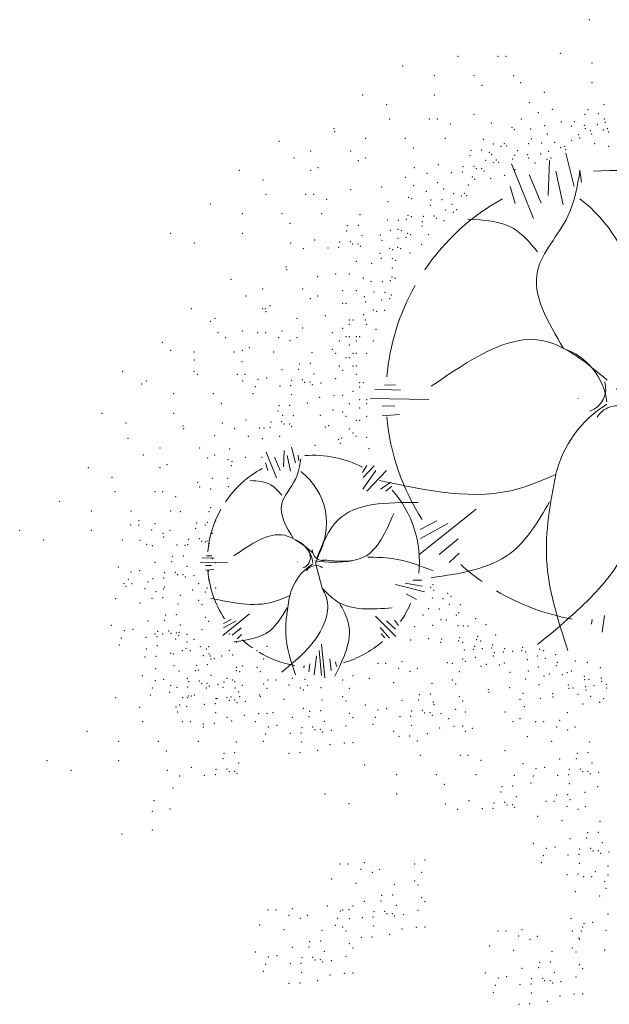
# Model space of a CAD drawing. Units: inches. Extents: x 1239 to 2276906, y 2273 to 321338.
# Tile 22 of 23: x 2267886 to 2272170, y 313785 to 320943. Entities that reach past the tile are written whole.
import ezdxf

# ---------------------------------------------------------------- set-up
doc = ezdxf.new("R2010")
doc.units = ezdxf.units.IN
doc.layers.add('L-PLNT', color=94, linetype='Continuous', lineweight=13)

# ---------------------------------------------------------------- blocks, each defined once
blk = doc.blocks.new('A$C30B31857')
for p, q in [((2.9834, 4.9924), (2.9378, 5.171)), ((2.7648, 4.82), (2.6466, 5.1137)), ((2.8434, 4.944), (2.8514, 5.1313)), ((2.8062, 4.9013), (2.7413, 5.0568)), ((2.9247, 4.894), (2.8853, 5.0751)), ((3.0223, 5.0135), (3.0144, 5.0799)), ((2.6661, 4.9009), (2.6393, 4.9915)), ((1.9621, 3.9222), (2.0223, 3.9241)), ((1.9103, 3.9012), (2.0497, 3.8956)), ((1.8883, 3.8498), (2.2022, 3.8449)), ((1.9494, 3.7571), (2.0441, 3.7647)), ((1.9499, 3.8105), (2.0188, 3.8098)), ((1.3819, 3.4241), (1.3265, 3.5618)), ((1.4188, 3.4822), (1.4225, 3.57)), ((1.4844, 3.5049), (1.463, 3.5887)), ((1.3356, 3.462), (1.3231, 3.5045)), ((1.4013, 3.4622), (1.3709, 3.5351)), ((1.4568, 3.4588), (1.4384, 3.5437)), ((1.5026, 3.5148), (1.4989, 3.546)), ((1.8439, 3.4518), (1.8684, 3.4899)), ((1.847, 3.3622), (1.9166, 3.4632)), ((1.8485, 3.4247), (1.9067, 3.4887)), ((1.868, 3.352), (1.973, 3.4627)), ((1.9418, 3.3622), (1.9966, 3.3999)), ((1.9699, 3.3518), (2.0024, 3.3789)), ((2.1467, 3.0086), (2.4563, 3.255)), ((2.1542, 3.1461), (2.2449, 3.1926)), ((2.1561, 3.097), (2.3032, 3.1772)), ((1.594, 2.9655), (1.6381, 3.0897)), ((2.2561, 3.01), (2.3583, 3.095)), ((0.971, 2.9694), (1.1182, 2.967)), ((0.9814, 2.9934), (1.0467, 2.9908)), ((1.0056, 3.0033), (1.0339, 3.0042)), ((2.3116, 2.9682), (2.3637, 3.0175)), ((0.9997, 2.9259), (1.0441, 2.9295)), ((0.9999, 2.9509), (1.0322, 2.9506)), ((1.5913, 2.9655), (1.6271, 2.8302)), ((2.1639, 2.8721), (2.1155, 2.8726)), ((2.1774, 2.8094), (2.0226, 2.8493)), ((2.1665, 2.8407), (2.0739, 2.8568)), ((2.1347, 2.7684), (2.0785, 2.7983)), ((1.0922, 2.575), (1.2373, 2.6905)), ((1.0957, 2.6395), (1.1382, 2.6613)), ((1.0966, 2.6164), (1.1655, 2.6541)), ((2.0239, 2.569), (1.9137, 2.6778)), ((2.0211, 2.6094), (1.9743, 2.6542)), ((2.0385, 2.6282), (2.0167, 2.6578)), ((3.0763, 2.6357), (3.0809, 2.6614)), ((3.1343, 2.5921), (3.1456, 2.6823)), ((1.1434, 2.5757), (1.1913, 2.6155)), ((1.9903, 2.5593), (1.9397, 2.6182)), ((1.1695, 2.5561), (1.1939, 2.5792)), ((1.9642, 2.5615), (1.9442, 2.5828)), ((1.6235, 2.359), (1.6107, 2.4933)), ((1.6415, 2.3458), (1.624, 2.5274)), ((1.584, 2.3634), (1.5971, 2.4652)), ((1.675, 2.3867), (1.6687, 2.4492)), ((1.5279, 2.4002), (1.5301, 2.4123)), ((1.5551, 2.3798), (1.5604, 2.4221)), ((1.7046, 2.4077), (1.6996, 2.4328))]:
    blk.add_line(p, q)
for centre, radius, start, end in [((3.1873, 3.861), 1.217, 62.402, 94.6709), ((3.1873, 3.861), 1.217, 118.935, 145.868), ((2.5377, 4.3028), 0.7844, 329.0782, 52.6009), ((3.1873, 3.861), 1.217, 150.5954, 174.9599), ((2.8122, 3.7899), 0.3494, 6.8841, 70.9351), ((3.0261, 3.9032), 0.1272, 289.2154, 17.1317), ((3.4797, 3.2971), 0.6129, 121.5433, 166.6017), ((3.1338, 3.8505), 0.1272, 179.4366, 180.2669), ((3.2157, 3.6838), 0.1272, 52.7337, 148.3189), ((3.1873, 3.861), 1.217, 185.1155, 212.961), ((1.58, 2.9746), 0.5705, 62.402, 94.6709), ((1.58, 2.9746), 0.5705, 118.935, 145.868), ((1.2979, 3.1775), 0.353, 329.0782, 52.6009), ((1.58, 2.9746), 0.5705, 353.5054, 42.0912), ((1.58, 2.9746), 0.5705, 150.5954, 174.9599), ((1.4214, 2.9466), 0.1572, 6.8841, 70.9351), ((1.633, 3.0374), 0.0596, 180.2669, 289.2154), ((1.5549, 2.9697), 0.0596, 179.4366, 180.2669), ((1.5044, 2.9943), 0.0596, 289.2154, 17.1317), ((1.6891, 3.6438), 0.6749, 261.4278, 278.5722), ((1.58, 2.9746), 0.5705, 185.1155, 212.961), ((1.7218, 2.7249), 0.2758, 121.5433, 166.6017), ((1.5933, 2.8915), 0.0596, 52.7337, 148.3189), ((3.1873, 3.861), 1.217, 227.9939, 234.9207), ((3.1873, 3.861), 1.217, 239.2549, 259.861), ((1.58, 2.9746), 0.5705, 325.3181, 336.4192), ((1.58, 2.9746), 0.5705, 227.9939, 234.9207), ((1.58, 2.9746), 0.5705, 286.5005, 310.702), ((1.58, 2.9746), 0.5705, 239.2549, 259.861)]:
    blk.add_arc(centre, radius, start, end)
for points, knots in [([(2.9263, 4.1201), (2.841, 4.2637), (2.6905, 4.5171), (2.9681, 4.7985), (3.0006, 4.9937), (3.0146, 5.0775)], [0, 0, 0, 0, 0.440566, 0.777274, 1.031196, 1.031196, 1.031196, 1.031196]), ([(2.7862, 4.6403), (2.7459, 4.6888), (2.6503, 4.8039), (2.4983, 4.8115), (2.4103, 4.8158)], [0, 0, 0, 0, 0.1819315, 0.4317682, 0.4317682, 0.4317682, 0.4317682]), ([(3.1616, 3.9488), (3.0492, 4.0429), (2.7553, 4.2891), (2.4209, 4.0585), (2.2144, 3.9161)], [0, 0, 0, 0, 0.40354, 1.055721, 1.055721, 1.055721, 1.055721]), ([(1.4728, 3.0952), (1.4344, 3.1599), (1.3667, 3.2739), (1.4916, 3.4005), (1.5062, 3.4883), (1.5125, 3.5261)], [0, 0, 0, 0, 0.1982546, 0.3497731, 0.4640382, 0.4640382, 0.4640382, 0.4640382]), ([(3.2693, 3.5312), (3.2945, 3.4812), (3.355, 3.361), (3.2868, 2.9371), (3.0051, 2.7057), (2.786, 2.5256)], [0, 0, 0, 0, 0.165135, 0.396758, 1.208872, 1.208872, 1.208872, 1.208872]), ([(1.4097, 3.3293), (1.3916, 3.3512), (1.3486, 3.403), (1.2802, 3.4063), (1.2406, 3.4083)], [0, 0, 0, 0, 0.0818692, 0.1942957, 0.1942957, 0.1942957, 0.1942957]), ([(2.884, 3.4417), (2.819, 3.4131), (2.522, 3.2824), (2.1934, 3.3535), (1.9367, 3.409)], [0, 0, 0, 0, 0.2107352, 0.9627078, 0.9627078, 0.9627078, 0.9627078]), ([(2.884, 3.4417), (2.8554, 3.2883), (2.7956, 2.967), (2.8966, 2.6556), (2.9493, 2.4929)], [0, 0, 0, 0, 0.4606481, 0.9645387, 0.9645387, 0.9645387, 0.9645387]), ([(1.6007, 2.9961), (1.6311, 3.0708), (1.7211, 3.2914), (1.9759, 3.2909), (2.1445, 3.2905)], [0, 0, 0, 0, 0.2272785, 0.6713114, 0.6713114, 0.6713114, 0.6713114]), ([(2.8513, 3.2945), (2.7895, 3.1889), (2.6492, 2.9493), (2.3704, 2.9084), (2.2144, 2.8855)], [0, 0, 0, 0, 0.3498703, 0.7941952, 0.7941952, 0.7941952, 0.7941952]), ([(1.6301, 2.9813), (1.7105, 2.9741), (1.8949, 2.9574), (1.9699, 3.1328), (2.0122, 3.2316)], [0, 0, 0, 0, 0.2209637, 0.5066723, 0.5066723, 0.5066723, 0.5066723]), ([(1.5786, 3.0182), (1.5281, 3.0605), (1.3958, 3.1713), (1.2454, 3.0675), (1.1524, 3.0034)], [0, 0, 0, 0, 0.1815929, 0.4750743, 0.4750743, 0.4750743, 0.4750743]), ([(1.8726, 2.9961), (1.917, 2.9955), (2.0386, 2.9939), (2.1529, 2.9502), (2.2254, 2.9225)], [0, 0, 0, 0, 0.132489, 0.3627011, 0.3627011, 0.3627011, 0.3627011]), ([(1.6271, 2.8302), (1.6384, 2.8077), (1.6657, 2.7536), (1.635, 2.5629), (1.5082, 2.4587), (1.4096, 2.3777)], [0, 0, 0, 0, 0.0743107, 0.1785413, 0.5439924, 0.5439924, 0.5439924, 0.5439924]), ([(1.6271, 2.8302), (1.6515, 2.8046), (1.7474, 2.7036), (1.8949, 2.7151), (2.0049, 2.7237)], [0, 0, 0, 0, 0.1034892, 0.4070428, 0.4070428, 0.4070428, 0.4070428]), ([(1.4537, 2.79), (1.4245, 2.7771), (1.2909, 2.7183), (1.143, 2.7503), (1.0275, 2.7752)], [0, 0, 0, 0, 0.0948308, 0.4332185, 0.4332185, 0.4332185, 0.4332185]), ([(1.4537, 2.79), (1.4409, 2.7209), (1.414, 2.5763), (1.4594, 2.4362), (1.4831, 2.363)], [0, 0, 0, 0, 0.2072917, 0.4340424, 0.4340424, 0.4340424, 0.4340424]), ([(1.439, 2.7237), (1.4112, 2.6762), (1.3481, 2.5684), (1.2226, 2.55), (1.1524, 2.5397)], [0, 0, 0, 0, 0.1574416, 0.3573878, 0.3573878, 0.3573878, 0.3573878]), ([(1.7183, 2.7531), (1.7397, 2.7142), (1.8095, 2.5877), (1.7426, 2.4506), (1.6962, 2.3556)], [0, 0, 0, 0, 0.1285246, 0.4177469, 0.4177469, 0.4177469, 0.4177469])]:
    blk.add_open_spline(points, degree=3, knots=knots)
for p in [(3.0641, 5.8899), (2.3591, 5.6932), (2.573, 5.6932), (2.6157, 5.6932), (2.9089, 5.7085), (2.0597, 5.641), (3.08, 5.6562), (2.2308, 5.5888), (2.4447, 5.5888), (2.6585, 5.5888), (2.4874, 5.5365), (2.695, 5.5518), (3.08, 5.5518), (1.8458, 5.4843), (2.2308, 5.4843), (2.8233, 5.4996), (1.9741, 5.4321), (2.7419, 5.4438), (3.1439, 5.4325), (1.99, 5.3551), (2.2039, 5.3551), (2.2466, 5.3551), (2.4447, 5.3798), (2.6996, 5.3561), (2.7913, 5.389), (2.8662, 5.4068), (3.0424, 5.3801), (3.0582, 5.4047), (3.1125, 5.3835), (3.1453, 5.3553), (1.6906, 5.3028), (2.3163, 5.3276), (2.5373, 5.3341), (2.6493, 5.3108), (2.749, 5.3012), (2.8239, 5.319), (2.9138, 5.3383), (2.9681, 5.3172), (2.9838, 5.3417), (3.0381, 5.3205), (3.0438, 5.303), (3.1081, 5.3239), (3.151, 5.3378), (3.1624, 5.3027), (1.6946, 5.2876), (1.8617, 5.2506), (2.0755, 5.2506), (2.2894, 5.2506), (2.6617, 5.2971), (2.8395, 5.2754), (3.0066, 5.2715), (3.0123, 5.2539), (3.071, 5.2924), (3.0767, 5.2748), (3.141, 5.2957), (3.1681, 5.2851), (1.3952, 5.2354), (2.1183, 5.1984), (2.495, 5.2464), (2.5488, 5.2203), (2.5903, 5.208), (2.607, 5.223), (2.607, 5.223), (2.6194, 5.2093), (2.738, 5.223), (2.7537, 5.2475), (2.808, 5.2263), (2.878, 5.2297), (2.9109, 5.2015), (2.9323, 5.2085), (2.9323, 5.2085), (2.9695, 5.24), (3.0938, 5.2222), (3.1695, 5.208), (1.4767, 5.1462), (1.5663, 5.1831), (1.7801, 5.1831), (1.8617, 5.1462), (2.4236, 5.1572), (2.428, 5.186), (2.4862, 5.1888), (2.5277, 5.1764), (2.54, 5.1627), (2.6636, 5.16), (2.6794, 5.1845), (2.7336, 5.1634), (2.7393, 5.1458), (2.8037, 5.1667), (2.8465, 5.1806), (2.8579, 5.1455), (2.938, 5.191), (1.605, 5.0939), (1.8229, 5.1309), (2.1231, 5.0932), (2.2518, 5.1099), (2.3857, 5.0983), (2.4439, 5.101), (2.5065, 5.1325), (2.548, 5.1202), (2.5647, 5.1353), (2.5771, 5.1216), (2.652, 5.1394), (2.7722, 5.1177), (2.8365, 5.1386), (1.1813, 5.0787), (1.5663, 5.0787), (2.0755, 5.0417), (2.1906, 5.0632), (2.3231, 5.0667), (2.3813, 5.0695), (2.4351, 5.0434), (2.4562, 5.0873), (2.4853, 5.0887), (2.4977, 5.0749), (2.6097, 5.0516), (2.665, 5.0828), (1.3096, 5.0264), (1.9472, 4.9895), (2.1202, 4.9958), (2.2488, 5.0125), (2.4139, 4.9995), (2.4474, 5.0297), (2.5347, 5.0338), (1.3255, 4.9494), (1.5393, 4.9494), (1.5821, 4.9494), (1.7801, 4.9742), (2.0927, 4.934), (2.1876, 4.9658), (2.2808, 4.979), (2.3346, 4.9529), (2.376, 4.9406), (2.3928, 4.9556), (2.3928, 4.9556), (2.4051, 4.9419), (1.0261, 4.8972), (1.6518, 4.922), (1.9809, 4.9098), (2.1095, 4.9265), (2.2094, 4.8898), (2.2138, 4.9186), (2.272, 4.9214), (2.3258, 4.8953), (1.1972, 4.845), (1.411, 4.845), (1.6249, 4.845), (1.8305, 4.8407), (2.0897, 4.8366), (2.0897, 4.8366), (2.1066, 4.8291), (2.1715, 4.8309), (2.2297, 4.8336), (2.2923, 4.8651), (2.3337, 4.8528), (2.3505, 4.8679), (1.4538, 4.7928), (1.7635, 4.7804), (1.8217, 4.7831), (1.9779, 4.8124), (2.0376, 4.8104), (2.0805, 4.816), (2.1648, 4.7785), (2.167, 4.8021), (2.242, 4.8199), (2.2835, 4.8075), (0.8122, 4.7405), (1.1972, 4.7405), (1.7591, 4.7516), (1.842, 4.7269), (1.9412, 4.73), (1.9933, 4.7562), (2.0362, 4.7618), (2.053, 4.7542), (2.0776, 4.7186), (2.0868, 4.7392), (2.1036, 4.7317), (2.1997, 4.7321), (0.9405, 4.6883), (1.4586, 4.6875), (1.5873, 4.7043), (1.7212, 4.6926), (1.7794, 4.6954), (1.7917, 4.6817), (1.8208, 4.683), (1.8332, 4.6693), (1.9489, 4.7019), (2.0347, 4.7131), (2.1619, 4.6811), (1.526, 4.6575), (1.6586, 4.6611), (1.7168, 4.6638), (1.9383, 4.6326), (1.9903, 4.6588), (2.0072, 4.6513), (2.0332, 4.6644), (2.0501, 4.6569), (2.1007, 4.6343), (1.4322, 4.5592), (1.8112, 4.5888), (1.8939, 4.5783), (1.946, 4.6045), (2.0057, 4.6026), (2.0226, 4.5951), (1.4362, 4.5439), (1.6032, 4.507), (1.7005, 4.5212), (1.7743, 4.5212), (2.0042, 4.5539), (1.1367, 4.4917), (1.8481, 4.4986), (1.8909, 4.4809), (1.9507, 4.479), (1.9936, 4.4846), (2.0028, 4.5052), (2.0028, 4.5052), (2.0196, 4.4977), (1.2183, 4.4025), (1.3078, 4.4395), (1.5217, 4.4395), (1.6032, 4.4025), (1.7374, 4.431), (1.8112, 4.431), (1.9063, 4.4247), (1.9661, 4.4228), (1.9998, 4.4078), (1.3466, 4.3503), (1.5645, 4.3872), (1.7374, 4.3634), (1.7558, 4.3634), (1.8543, 4.3986), (1.862, 4.3705), (1.9477, 4.3816), (1.9906, 4.3872), (0.9229, 4.335), (1.3078, 4.335), (1.3214, 4.3338), (1.3254, 4.3186), (1.6451, 4.2957), (1.8513, 4.3012), (1.9034, 4.3274), (1.9202, 4.3199), (1.9631, 4.3254), (1.026, 4.2664), (1.0512, 4.2828), (1.4925, 4.2816), (1.7743, 4.2732), (1.7743, 4.2732), (1.7743, 4.2506), (1.7928, 4.2732), (1.859, 4.2731), (1.8666, 4.2506), (1.0671, 4.2058), (1.1971, 4.2141), (1.2809, 4.2058), (1.3237, 4.2058), (1.411, 4.2141), (1.5217, 4.2306), (1.682, 4.2056), (1.7374, 4.2281), (1.9173, 4.2225), (0.7676, 4.1536), (1.1075, 4.1772), (1.3934, 4.1783), (1.4537, 4.1619), (1.4925, 4.1772), (1.7189, 4.1605), (1.7558, 4.183), (1.7743, 4.183), (1.7743, 4.1379), (1.8112, 4.183), (1.8112, 4.1605), (1.8297, 4.183), (1.9035, 4.1605), (0.8121, 4.1097), (0.9387, 4.1013), (1.1526, 4.1013), (1.1971, 4.1097), (1.2359, 4.1249), (1.3665, 4.1013), (1.5721, 4.0971), (1.682, 4.1154), (1.7005, 4.0929), (1.7928, 4.0929), (1.8112, 4.0929), (1.8666, 4.0929), (0.9404, 4.0574), (1.1954, 4.0491), (1.5051, 4.0368), (1.5633, 4.0395), (1.7558, 4.0703), (1.7743, 4.0703), (0.5538, 3.9969), (0.9387, 3.9969), (0.9563, 3.9804), (1.1702, 3.9804), (1.2129, 3.9804), (1.411, 4.0052), (1.5007, 4.008), (1.5836, 3.9833), (1.7189, 4.0252), (1.7374, 4.0027), (1.7928, 4.0252), (1.8112, 4.0252), (1.8112, 3.9801), (0.6569, 3.9282), (0.6821, 3.9447), (1.2002, 3.9439), (1.2826, 3.953), (1.3289, 3.9606), (1.4628, 3.949), (1.521, 3.9517), (1.5333, 3.938), (1.5624, 3.9394), (1.5748, 3.9257), (1.6207, 3.9335), (1.7005, 3.9576), (1.8297, 3.9351), (1.8297, 3.9351), (1.8481, 3.9351), (0.828, 3.876), (1.0418, 3.876), (1.2557, 3.876), (1.2676, 3.9139), (1.4001, 3.9175), (1.4583, 3.9202), (1.4613, 3.8717), (1.7928, 3.89), (1.8297, 3.9125), (1.0846, 3.8238), (1.547, 3.8267), (1.6145, 3.8567), (1.6911, 3.8661), (1.7374, 3.8674), (1.7743, 3.8223), (1.8297, 3.8449), (1.8666, 3.8449), (1.8666, 3.8223), (0.443, 3.7715), (0.828, 3.7715), (1.3899, 3.7826), (1.3943, 3.8114), (1.4525, 3.8141), (1.6849, 3.7894), (1.7374, 3.7773), (1.8297, 3.7998), (0.5713, 3.7193), (1.0894, 3.7186), (1.2181, 3.7353), (1.352, 3.7236), (1.4102, 3.7264), (1.4147, 3.7591), (1.4226, 3.7127), (1.4517, 3.714), (1.4728, 3.7579), (1.6174, 3.7593), (1.7558, 3.7547), (1.8112, 3.7322), (1.8297, 3.7322), (1.8666, 3.7547), (0.8784, 3.7029), (0.8824, 3.6876), (1.1569, 3.6885), (1.2894, 3.6921), (1.3136, 3.6915), (1.3476, 3.6948), (1.464, 3.7003), (1.6449, 3.6975), (1.6618, 3.7051), (1.7743, 3.6871), (1.7928, 3.6645), (0.583, 3.6354), (1.0495, 3.6506), (1.2301, 3.6464), (1.3048, 3.6339), (1.3994, 3.6464), (1.7153, 3.6302), (1.7153, 3.6302), (1.7245, 3.6096), (1.7322, 3.6377), (1.8088, 3.6471), (1.8666, 3.642), (0.7541, 3.5832), (0.9679, 3.5832), (1.1291, 3.5788), (1.5881, 3.5982), (1.8792, 3.5798), (0.6645, 3.5462), (1.0107, 3.5309), (1.0495, 3.5462), (1.1203, 3.5212), (1.1417, 3.5118), (1.2148, 3.5337), (1.304, 3.5338), (0.3691, 3.4787), (0.7541, 3.4787), (0.7928, 3.494), (1.1379, 3.4887), (0.4974, 3.4265), (0.9571, 3.3992), (1.0368, 3.4211), (1.1194, 3.4211), (0.5133, 3.3495), (0.7272, 3.3495), (0.7699, 3.3495), (0.9679, 3.3742), (1.028, 3.3635), (1.1225, 3.376), (0.2139, 3.2972), (0.8396, 3.322), (0.385, 3.245), (0.5988, 3.245), (0.8127, 3.245), (0.8648, 3.2414), (1.0183, 3.2408), (1.0271, 3.2633), (0.6416, 3.1928), (1.0095, 3.1832), (1.0544, 3.1915), (0, 3.1406), (0.385, 3.1406), (0.5979, 3.1692), (0.6407, 3.1692), (0.7104, 3.1417), (0.728, 3.1775), (0.8095, 3.1406), (0.9469, 3.1516), (0.9513, 3.1804), (0.999, 3.169), (0.1283, 3.0883), (0.5529, 3.0883), (0.6464, 3.0876), (0.7708, 3.1253), (0.7751, 3.1043), (0.909, 3.0927), (0.9672, 3.0954), (0.9795, 3.0817), (0.999, 3.0788), (1.0086, 3.0831), (1.0298, 3.1269), (1.036, 3.1239), (0.6835, 3.0647), (0.7139, 3.0576), (0.8464, 3.0611), (0.8891, 3.0605), (0.9046, 3.0639), (1.0175, 3.0562), (1.021, 3.0693), (0.728, 2.9686), (0.8177, 2.9714), (0.8221, 3.0002), (0.8803, 3.0029), (1.036, 2.9886), (0.53, 2.9438), (0.5997, 2.9164), (0.6459, 2.924), (0.9006, 2.9467), (1.0175, 2.921), (1.0544, 2.9661), (0.5846, 2.8773), (0.7172, 2.8809), (0.7754, 2.8836), (0.7798, 2.9124), (0.838, 2.9151), (0.8503, 2.9014), (0.8794, 2.9028), (0.8918, 2.8891), (0.9377, 2.8969), (1.0175, 2.876), (0.561, 2.8537), (0.5727, 2.8394), (0.6038, 2.8537), (0.6735, 2.8262), (0.6911, 2.862), (0.7338, 2.8098), (0.7726, 2.8251), (0.7783, 2.8351), (0.9315, 2.8201), (0.9621, 2.8535), (1.0081, 2.8295), (1.0544, 2.8308), (2.2113, 2.8337), (2.2113, 2.8337), (2.2237, 2.8474), (2.2281, 2.8186), (0.516, 2.7728), (0.7113, 2.7748), (0.7695, 2.7775), (0.864, 2.7901), (0.9621, 2.7633), (0.999, 2.8084), (2.2201, 2.7761), (2.2783, 2.7733), (2.303, 2.8008), (2.3198, 2.7857), (0.6466, 2.7492), (0.8522, 2.745), (0.9806, 2.7408), (2.1998, 2.7198), (2.258, 2.7171), (2.3118, 2.7432), (2.37, 2.7404), (0.6911, 2.6531), (0.7808, 2.6559), (0.7852, 2.6847), (0.8434, 2.6874), (0.999, 2.6731), (1.0175, 2.6506), (2.1698, 2.6846), (2.2668, 2.6595), (2.2959, 2.6581), (2.3497, 2.6842), (2.3621, 2.6979), (2.4538, 2.665), (0.4931, 2.6284), (0.5627, 2.6009), (0.609, 2.6086), (0.8011, 2.5996), (0.8637, 2.6312), (0.9806, 2.6055), (1.1836, 2.6056), (2.1255, 2.6213), (2.2227, 2.6286), (2.3585, 2.6266), (2.3876, 2.6252), (2.4113, 2.6255), (2.5085, 2.6327), (0.5477, 2.5618), (0.6803, 2.5654), (0.7272, 2.5833), (0.7385, 2.5681), (0.7429, 2.5969), (0.7699, 2.5833), (0.8134, 2.5859), (0.8396, 2.5558), (0.8425, 2.5873), (0.8549, 2.5736), (0.8572, 2.5916), (0.9008, 2.5814), (0.9387, 2.5547), (1.1283, 2.5831), (2.1027, 2.5511), (2.1999, 2.5584), (2.2699, 2.555), (2.3614, 2.5447), (2.3614, 2.5447), (2.3671, 2.5623), (2.4585, 2.5519), (2.4642, 2.5695), (2.48, 2.545), (2.5614, 2.5767), (0.5358, 2.5239), (0.6821, 2.5024), (0.7414, 2.5197), (0.8748, 2.4932), (0.8946, 2.5046), (0.9, 2.5394), (0.9176, 2.4932), (0.9712, 2.5141), (1.0049, 2.5015), (1.0175, 2.5153), (1.1283, 2.4929), (1.1652, 2.538), (1.2759, 2.4929), (1.3313, 2.5155), (2.2642, 2.5375), (2.3828, 2.5377), (2.3928, 2.4957), (2.4414, 2.4993), (2.4471, 2.5168), (2.49, 2.5029), (2.5386, 2.5065), (2.5443, 2.5241), (2.6086, 2.5032), (2.7001, 2.4929), (2.7001, 2.4929), (2.7058, 2.5104), (2.7972, 2.5001), (2.8187, 2.4931), (0.6744, 2.4593), (0.7326, 2.4621), (0.8127, 2.4788), (0.8271, 2.4746), (0.9873, 2.4657), (1.0183, 2.4746), (1.0261, 2.4635), (1.0301, 2.4482), (1.0476, 2.4493), (1.0864, 2.4645), (1.1467, 2.4703), (1.3128, 2.4478), (2.3834, 2.4479), (2.4514, 2.4572), (2.5486, 2.4645), (2.5543, 2.482), (2.6029, 2.4856), (2.6515, 2.4892), (2.7215, 2.4859), (2.7315, 2.4438), (2.7858, 2.465), (2.8287, 2.4511), (2.883, 2.4722), (0.7307, 2.396), (0.8298, 2.4123), (0.9469, 2.3855), (0.9513, 2.4143), (0.9604, 2.3887), (1.0095, 2.417), (1.1652, 2.4027), (1.1972, 2.4112), (1.2759, 2.4027), (1.6362, 2.407), (1.927, 2.4255), (1.9698, 2.4255), (2.0394, 2.3981), (2.057, 2.4339), (2.1386, 2.3969), (2.3, 2.4288), (2.3281, 2.4253), (2.3972, 2.436), (2.4829, 2.4082), (2.5101, 2.4188), (2.5801, 2.4154), (2.6072, 2.426), (2.7901, 2.4054), (2.8873, 2.4126), (2.893, 2.4302), (2.9902, 2.4374), (3.0533, 2.4302), (3.1244, 2.4005), (0.6592, 2.3579), (0.7751, 2.3381), (0.8572, 2.3827), (0.9017, 2.3437), (1.0298, 2.3608), (1.1156, 2.3437), (1.1467, 2.3351), (1.166, 2.3844), (1.1836, 2.3802), (1.2944, 2.3802), (1.3363, 2.3354), (1.3791, 2.3354), (1.4663, 2.3437), (1.5352, 2.3394), (1.7374, 2.3352), (1.7928, 2.3577), (1.8819, 2.3447), (2.0998, 2.3816), (2.3281, 2.3351), (2.365, 2.3802), (2.6387, 2.377), (2.7228, 2.3398), (2.7359, 2.3842), (2.8216, 2.3563), (2.8488, 2.3669), (2.9188, 2.3636), (2.9459, 2.3742), (2.9674, 2.384), (3.0386, 2.3544), (3.0405, 2.336), (3.0629, 2.3384), (3.1302, 2.3455), (0.7139, 2.2914), (0.7289, 2.3305), (0.8122, 2.3068), (0.8464, 2.2949), (0.9046, 2.2977), (0.909, 2.3265), (0.9672, 2.3292), (0.9795, 2.3155), (1.0049, 2.2926), (1.0086, 2.3169), (1.021, 2.3032), (1.0669, 2.311), (1.0946, 2.2953), (1.099, 2.3241), (1.1572, 2.3268), (1.1584, 2.2915), (1.1972, 2.3068), (1.3128, 2.3126), (1.3313, 2.29), (1.4488, 2.3079), (1.5091, 2.2915), (1.5263, 2.2818), (1.5479, 2.3068), (1.6209, 2.2943), (1.7743, 2.2901), (2.0125, 2.3211), (2.2181, 2.3168), (2.3465, 2.3126), (2.5212, 2.2832), (2.6369, 2.2936), (2.7939, 2.3101), (2.9527, 2.3083), (2.9547, 2.2899), (2.9547, 2.2899), (2.9771, 2.2923), (3.0443, 2.2993), (3.0463, 2.281), (3.0892, 2.3041), (3.1321, 2.3271), (3.1564, 2.3111), (3.1584, 2.2928), (0.5168, 2.2393), (0.702, 2.2535), (0.8069, 2.2678), (0.8765, 2.2403), (0.9017, 2.2393), (0.9076, 2.2492), (0.9228, 2.248), (0.9405, 2.2545), (1.0567, 2.2363), (1.0607, 2.2342), (1.1149, 2.2391), (1.1373, 2.2436), (1.1563, 2.2267), (1.1775, 2.2706), (1.1836, 2.2449), (1.2912, 2.2545), (1.2944, 2.2449), (1.4218, 2.2309), (1.6274, 2.2267), (1.7374, 2.245), (2.1467, 2.2277), (2.1511, 2.2565), (2.2093, 2.2592), (2.365, 2.245), (2.5252, 2.2679), (2.6923, 2.2309), (2.7081, 2.264), (2.8016, 2.2367), (2.8669, 2.2621), (2.8689, 2.2438), (3.0034, 2.2579), (3.0726, 2.2466), (3.1417, 2.2353), (0.6451, 2.1871), (0.8405, 2.1889), (0.8615, 2.2012), (0.8987, 2.1916), (0.9933, 2.2042), (0.9941, 2.2048), (1.0523, 2.2075), (1.1272, 2.2254), (1.1687, 2.213), (1.2146, 2.2209), (1.5255, 2.1817), (1.7559, 2.2225), (1.859, 2.2002), (1.9749, 2.1804), (2.057, 2.225), (2.2258, 2.2157), (2.2296, 2.203), (2.3465, 2.1773), (2.3834, 2.2224), (2.7158, 2.1906), (3.0316, 2.2052), (3.1213, 2.2146), (0.8496, 2.1633), (1.0552, 2.1591), (1.1156, 2.1348), (1.2084, 2.1441), (1.285, 2.1535), (1.3313, 2.1548), (1.3632, 2.1597), (1.4663, 2.1348), (1.556, 2.1376), (1.5604, 2.1664), (1.6186, 2.1691), (1.7743, 2.1548), (1.7928, 2.1323), (1.9137, 2.1336), (1.9287, 2.1727), (2.0462, 2.1372), (2.1044, 2.1399), (2.1088, 2.1687), (2.167, 2.1715), (2.1794, 2.1578), (2.2085, 2.1591), (2.2208, 2.1454), (2.2667, 2.1533), (2.3074, 2.1265), (2.3969, 2.1635), (2.6108, 2.1635), (2.6923, 2.1265), (2.9458, 2.1591), (0.661, 2.1101), (0.8748, 2.1101), (0.9176, 2.1101), (0.9873, 2.0826), (0.9882, 2.0988), (1.0464, 2.1015), (1.1409, 2.114), (1.2683, 2.1101), (1.338, 2.0826), (1.3842, 2.0903), (1.5181, 2.0786), (1.5763, 2.0813), (1.5887, 2.0676), (1.6178, 2.069), (1.6389, 2.1129), (1.7559, 2.0872), (1.9018, 2.0957), (2.1074, 2.0915), (2.2605, 2.0765), (2.3371, 2.0859), (2.3834, 2.0872), (2.4357, 2.0743), (2.6536, 2.1112), (2.7761, 2.1101), (2.8189, 2.1101), (2.8886, 2.0826), (2.9061, 2.1184), (2.9877, 2.0814), (0.3615, 2.0578), (1.323, 2.0435), (1.4555, 2.0471), (1.5137, 2.0498), (1.6301, 2.0553), (1.6761, 2.0631), (2.0119, 2.059), (2.0404, 2.0312), (2.0986, 2.0339), (2.1931, 2.0464), (2.3969, 2.059), (2.731, 2.0292), (2.9489, 2.0662), (0.5326, 2.0056), (0.7465, 2.0056), (0.9604, 2.0056), (1.166, 2.0014), (1.3111, 2.0056), (1.5167, 2.0014), (1.6698, 1.9863), (1.7464, 1.9958), (1.7928, 1.997), (2.1403, 2.0068), (2.8616, 2.0056), (3.0672, 2.0014), (0.7893, 1.9534), (1.0946, 1.9122), (1.099, 1.941), (1.1572, 1.9438), (1.4497, 1.941), (1.5079, 1.9438), (1.6024, 1.9563), (2.1561, 1.9298), (2.37, 1.9298), (2.4128, 1.9298), (2.6108, 1.9545), (2.9061, 1.9095), (2.9958, 1.9122), (3.0002, 1.941), (3.0584, 1.9438), (0.1477, 1.9011), (0.5326, 1.9011), (0.9228, 1.8649), (1.1149, 1.856), (1.1775, 1.8875), (1.8567, 1.8776), (2.4825, 1.9023), (2.7081, 1.8847), (2.7778, 1.8572), (2.824, 1.8649), (3.0161, 1.856), (3.0787, 1.8875), (0.276, 1.8489), (0.7941, 1.8482), (0.8615, 1.8181), (0.9941, 1.8217), (1.0523, 1.8245), (1.0567, 1.8533), (1.1272, 1.8423), (1.1563, 1.8436), (1.1687, 1.8299), (2.0278, 1.8253), (2.2417, 1.8253), (2.4555, 1.8253), (2.6611, 1.8211), (2.7628, 1.8181), (2.8953, 1.8217), (2.9535, 1.8245), (2.9579, 1.8533), (3.0285, 1.8423), (3.0576, 1.8436), (3.0699, 1.8299), (3.1158, 1.8378), (0.8241, 1.7535), (2.2844, 1.7731), (2.5941, 1.7607), (2.6523, 1.7635), (2.7509, 1.7803), (2.9565, 1.776), (3.1096, 1.761), (1.6428, 1.7209), (2.0278, 1.7209), (2.5897, 1.7319), (2.6726, 1.7072), (2.8895, 1.7157), (2.9477, 1.7184), (3.0422, 1.731), (0.723, 1.6859), (1.7712, 1.6686), (2.2893, 1.6679), (2.4179, 1.6846), (2.5474, 1.6442), (2.5518, 1.673), (2.61, 1.6757), (2.6224, 1.662), (2.6515, 1.6634), (2.6638, 1.6497), (2.8315, 1.6819), (2.8742, 1.6819), (2.9439, 1.6544), (2.9615, 1.6902), (3.043, 1.6533), (0.7142, 1.6283), (0.8087, 1.6408), (2.3567, 1.6379), (2.4892, 1.6414), (2.7864, 1.601), (3.0043, 1.638), (2.917, 1.5774), (3.1226, 1.5732), (0.551, 1.5062), (0.7133, 1.5282), (3.0556, 1.5129), (3.1138, 1.5156), (2.7635, 1.4565), (2.8794, 1.4367), (2.9615, 1.4813), (3.0512, 1.4841), (3.1341, 1.4594), (2.8182, 1.39), (2.8332, 1.4291), (2.9507, 1.3936), (3.0089, 1.3963), (3.0133, 1.4251), (3.0715, 1.4278), (3.0838, 1.4141), (3.1129, 1.4155), (3.1253, 1.4018), (3.1712, 1.4096), (1.7239, 1.3439), (1.7667, 1.3439), (1.854, 1.3522), (2.125, 1.3436), (2.1804, 1.3662), (2.8063, 1.3521), (3.0119, 1.3478), (3.165, 1.3328), (1.8364, 1.3164), (1.8967, 1.3), (1.9355, 1.3152), (2.1619, 1.2986), (2.9448, 1.2875), (3.0031, 1.2902), (3.0345, 1.2763), (3.0773, 1.2763), (3.0976, 1.3028), (3.1645, 1.2846), (1.6789, 1.263), (1.8095, 1.2394), (2.0151, 1.2352), (2.125, 1.2535), (2.1435, 1.2309), (3.147, 1.2488), (1.9481, 1.1748), (2.0063, 1.1776), (2.9894, 1.1954), (3.1201, 1.1718), (3.1537, 1.2133), (1.656, 1.1185), (1.7928, 1.1183), (1.854, 1.1433), (1.9437, 1.146), (2.0266, 1.1213), (2.1619, 1.1633), (2.1804, 1.1408), (1.3363, 1.096), (1.3791, 1.096), (1.4488, 1.0685), (1.4663, 1.1043), (1.5479, 1.0674), (1.7256, 1.0911), (1.7374, 1.0958), (1.7719, 1.0987), (1.9058, 1.0871), (1.964, 1.0898), (1.9763, 1.0761), (2.0054, 1.0775), (2.0178, 1.0637), (2.0637, 1.0716), (2.1435, 1.0957), (3.1645, 1.0757), (1.2912, 1.0151), (1.5091, 1.0521), (1.6987, 1.0141), (1.7106, 1.052), (1.7743, 1.0507), (1.8432, 1.0555), (1.9014, 1.0583), (1.9043, 1.0098), (2.9665, 1.0509), (3.0362, 1.0235), (3.0824, 1.0311), (1.4218, 0.9915), (1.6274, 0.9873), (1.7374, 1.0056), (1.7559, 0.983), (1.99, 0.9648), (2.0575, 0.9948), (2.1341, 1.0042), (2.1804, 1.0055), (2.573, 0.9833), (2.6158, 0.9833), (2.6855, 0.9559), (2.7031, 0.9916), (2.7846, 0.9547), (2.9741, 0.9831), (3.0212, 0.9843), (3.0295, 1.0056), (3.1537, 0.9879), (1.5604, 0.927), (1.6186, 0.9297), (1.7743, 0.9154), (1.8373, 0.9495), (1.8955, 0.9522), (2.528, 0.9024), (2.7459, 0.9394), (3.0093, 0.9465), (3.011, 0.938), (1.2683, 0.8706), (1.3842, 0.8508), (1.4663, 0.8954), (1.556, 0.8982), (1.6389, 0.8735), (1.7928, 0.8929), (2.6586, 0.8789), (2.8642, 0.8746), (2.9741, 0.8929), (2.9926, 0.8704), (3.1479, 0.8819), (1.323, 0.8041), (1.338, 0.8432), (1.4555, 0.8076), (1.5137, 0.8104), (1.5181, 0.8392), (1.5763, 0.8419), (1.5887, 0.8282), (1.6178, 0.8296), (1.6301, 0.8159), (1.6761, 0.8237), (1.7559, 0.8478), (2.7972, 0.8143), (2.8554, 0.817), (3.011, 0.8027), (1.3111, 0.7662), (1.5167, 0.7619), (1.6698, 0.7469), (1.7464, 0.7563), (1.7928, 0.7576), (2.5051, 0.758), (2.7031, 0.7827), (2.7928, 0.7855), (2.8757, 0.7608), (3.0295, 0.7802), (1.4497, 0.7016), (1.5079, 0.7043), (1.6024, 0.7169), (2.5597, 0.6914), (2.5748, 0.7305), (2.621, 0.7382), (2.6923, 0.695), (2.7505, 0.6977), (2.7549, 0.7265), (2.8131, 0.7293), (2.8254, 0.7155), (2.8545, 0.7169), (2.8669, 0.7032), (2.9128, 0.711), (2.9926, 0.7351), (2.5478, 0.6535), (2.7534, 0.6493), (2.9832, 0.6437), (3.0295, 0.6449), (2.6864, 0.5889), (2.7446, 0.5917), (2.8391, 0.6042), (2.9066, 0.6342)]:
    blk.add_point(p)
blk = doc.blocks.new('p2')
at = {"xscale": 1000, "yscale": 1000, "zscale": 1000}
blk.add_blockref('A$C30B31857', (-714.2, -1628.3), dxfattribs=at)

msp = doc.modelspace()

# ---------------------------------------------------------------- block references
at = {"layer": 'L-PLNT', "xscale": 1.35042108782907, "yscale": 1.35042108782907, "zscale": 1.35042108782907}
msp.add_blockref('p2', (2268850.67, 315188.45), dxfattribs=at)

doc.saveas('drawing.dxf')
